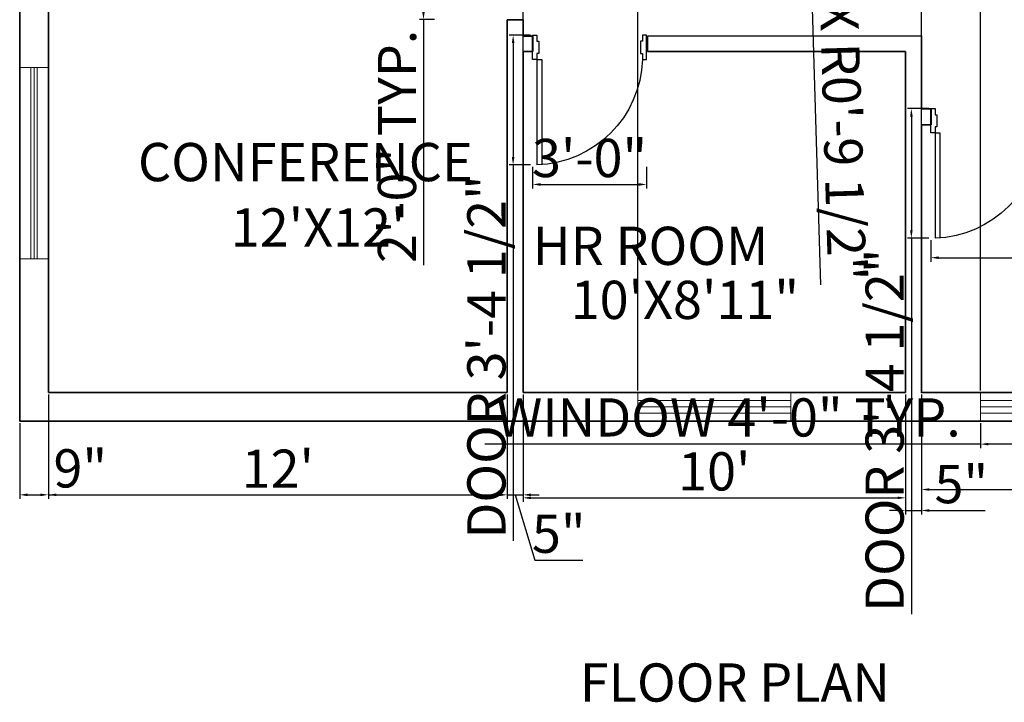
# Model space of a CAD drawing. Units: inches. Extents: x 2319 to 3765, y 2872 to 3950.
# Tile 2 of 9: x 2474 to 2783, y 2872 to 3087. Entities that reach past the tile are written whole.
import ezdxf

# ---------------------------------------------------------------- set-up
doc = ezdxf.new("R2010")
doc.units = ezdxf.units.IN
for name, color, linetype, lineweight in [('A-ANNO-DIMS', 2, 'Continuous', 18), ('A-ANNO-TEXT', 7, 'Continuous', 25), ('A-AREA-IDEN', 7, 'Continuous', 18), ('A-DOOR', 3, 'Continuous', 25), ('A-GLAZ', 4, 'Continuous', 18), ('A-WALL', 7, 'Continuous', 35)]:
    doc.layers.add(name, color=color, linetype=linetype, lineweight=lineweight)
doc.styles.get("Standard").update_dxf_attribs({"font": 'arial.ttf'})
doc.dimstyles.new('ISO-25', dxfattribs={"dimtxt": 12, "dimasz": 2.5, "dimexe": 1.25, "dimexo": 0.625, "dimtad": 1, "dimdec": 0, "dimlunit": 3, "dimtxsty": 'Standard', "dimcen": 2.5, "dimadec": 0, "dimazin": 0, "dimtfac": 1, "dimtdec": 0, "dimtmove": 0, "dimatfit": 3, "dimfxl": 1, "dimarcsym": 0})

# ---------------------------------------------------------------- blocks, each defined once
blk = doc.blocks.new('A$C769D55ED')
for p, q in [((33.6, 192), (33.6, 1024.8)), ((72, 192), (72, 1023.9)), ((0, 192), (0, 0)), ((33.6, 192), (0, 192)), ((33.6, 144), (33.6, 192)), ((48, 144), (33.6, 144)), ((48, 48), (48, 144)), ((33.6, 0), (33.6, 48)), ((33.6, 48), (48, 48)), ((0, 0), (33.6, 0))]:
    blk.add_line(p, q)
blk.add_lwpolyline([(33.6, 192), (72, 192)])
blk.add_lwpolyline([(900, 192), (900, 0), (866.4, 0), (866.4, 48), (852, 48), (852, 144), (866.4, 144), (866.4, 192)], close=True)
blk.add_arc((7.2, 165.6), 859.6, 1.76235, 88.23765)
blk = doc.blocks.new('*D20')
at = {"layer": 'A-ANNO-DIMS', "color": 0, "lineweight": -2, "transparency": 16777216}
for p, q in [((2483.13, 2968.99), (2483.13, 2936.24)), ((2627.13, 2968.99), (2627.13, 2936.24)), ((2485.63, 2937.49), (2624.63, 2937.49))]:
    blk.add_line(p, q, dxfattribs=at)
at = {"layer": 'A-ANNO-DIMS', "color": 0, "transparency": 16777216}
for points in [[(2485.63, 2937.91), (2485.63, 2937.07), (2483.13, 2937.49)], [(2624.63, 2937.91), (2624.63, 2937.07), (2627.13, 2937.49)]]:
    blk.add_solid(points, dxfattribs=at)
at = {"layer": 'Defpoints', "color": 0, "transparency": 16777216}
for p in [(2483.13, 2969.61), (2627.13, 2969.61), (2627.13, 2937.49)]:
    blk.add_point(p, dxfattribs=at)
at = {"layer": 'A-ANNO-DIMS', "color": 0, "transparency": 16777216, "insert": (2555.13, 2944.14), "char_height": 12, "attachment_point": 5}
blk.add_mtext("12'", dxfattribs=at)
blk = doc.blocks.new('*D21')
at = {"layer": 'A-ANNO-DIMS', "color": 0, "lineweight": -2, "transparency": 16777216}
for p, q in [((2632.13, 2968.99), (2632.13, 2935.3)), ((2752.13, 2968.99), (2752.13, 2935.3)), ((2634.63, 2936.55), (2749.63, 2936.55))]:
    blk.add_line(p, q, dxfattribs=at)
at = {"layer": 'A-ANNO-DIMS', "color": 0, "transparency": 16777216}
for points in [[(2634.63, 2936.96), (2634.63, 2936.13), (2632.13, 2936.55)], [(2749.63, 2936.96), (2749.63, 2936.13), (2752.13, 2936.55)]]:
    blk.add_solid(points, dxfattribs=at)
at = {"layer": 'Defpoints', "color": 0, "transparency": 16777216}
for p in [(2632.13, 2969.61), (2752.13, 2969.61), (2752.13, 2936.55)]:
    blk.add_point(p, dxfattribs=at)
at = {"layer": 'A-ANNO-DIMS', "color": 0, "transparency": 16777216, "insert": (2692.13, 2943.3), "char_height": 12, "attachment_point": 5}
blk.add_mtext("10'", dxfattribs=at)
blk = doc.blocks.new('*D22')
at = {"layer": 'A-ANNO-DIMS', "color": 0, "lineweight": -2, "transparency": 16777216}
for p, q in [((2757.13, 2968.99), (2757.13, 2937.91)), ((2946.13, 2968.99), (2946.13, 2937.91)), ((2759.63, 2939.16), (2943.63, 2939.16))]:
    blk.add_line(p, q, dxfattribs=at)
at = {"layer": 'A-ANNO-DIMS', "color": 0, "transparency": 16777216}
for points in [[(2759.63, 2939.58), (2759.63, 2938.74), (2757.13, 2939.16)], [(2943.63, 2939.58), (2943.63, 2938.74), (2946.13, 2939.16)]]:
    blk.add_solid(points, dxfattribs=at)
at = {"layer": 'Defpoints', "color": 0, "transparency": 16777216}
for p in [(2757.13, 2969.61), (2946.13, 2969.61), (2946.13, 2939.16)]:
    blk.add_point(p, dxfattribs=at)
at = {"layer": 'A-ANNO-DIMS', "color": 0, "transparency": 16777216, "insert": (2851.63, 2945.91), "char_height": 12, "attachment_point": 5}
blk.add_mtext('15\'-9"', dxfattribs=at)
blk = doc.blocks.new('*D23')
at = {"layer": 'A-ANNO-DIMS', "color": 0, "lineweight": -2, "transparency": 16777216}
for p, q in [((2474.13, 2959.99), (2474.13, 2936.24)), ((2483.13, 2951.99), (2483.13, 2936.24)), ((2476.63, 2937.49), (2480.63, 2937.49)), ((2483.13, 2937.49), (2500.67, 2937.49))]:
    blk.add_line(p, q, dxfattribs=at)
at = {"layer": 'A-ANNO-DIMS', "color": 0, "transparency": 16777216}
for points in [[(2476.63, 2937.91), (2476.63, 2937.07), (2474.13, 2937.49)], [(2480.63, 2937.91), (2480.63, 2937.07), (2483.13, 2937.49)]]:
    blk.add_solid(points, dxfattribs=at)
at = {"layer": 'Defpoints', "color": 0, "transparency": 16777216}
for p in [(2474.13, 2960.61), (2483.13, 2952.61), (2483.13, 2937.49)]:
    blk.add_point(p, dxfattribs=at)
at = {"layer": 'A-ANNO-DIMS', "color": 0, "transparency": 16777216, "insert": (2493.15, 2944.24), "char_height": 12, "attachment_point": 5}
blk.add_mtext('9"', dxfattribs=at)
blk = doc.blocks.new('*D24')
at = {"layer": 'A-ANNO-DIMS', "color": 0, "lineweight": -2, "transparency": 16777216}
for p, q in [((2627.13, 2968.99), (2627.13, 2936.24)), ((2632.13, 2968.99), (2632.13, 2936.24)), ((2624.63, 2937.49), (2622.13, 2937.49)), ((2627.13, 2937.49), (2632.13, 2937.49)), ((2627.13, 2937.49), (2632.13, 2937.49)), ((2629.63, 2937.49), (2635.78, 2916.99)), ((2634.63, 2937.49), (2637.13, 2937.49)), ((2635.78, 2916.99), (2650.82, 2916.99))]:
    blk.add_line(p, q, dxfattribs=at)
at = {"layer": 'A-ANNO-DIMS', "color": 0, "transparency": 16777216}
for points in [[(2624.63, 2937.91), (2624.63, 2937.07), (2627.13, 2937.49)], [(2634.63, 2937.91), (2634.63, 2937.07), (2632.13, 2937.49)]]:
    blk.add_solid(points, dxfattribs=at)
at = {"layer": 'Defpoints', "color": 0, "transparency": 16777216}
for p in [(2627.13, 2969.61), (2632.13, 2969.61), (2632.13, 2937.49)]:
    blk.add_point(p, dxfattribs=at)
at = {"layer": 'A-ANNO-DIMS', "color": 0, "transparency": 16777216, "insert": (2643.3, 2923.72), "char_height": 12, "attachment_point": 5}
blk.add_mtext('5"', dxfattribs=at)
blk = doc.blocks.new('*D25')
at = {"layer": 'A-ANNO-DIMS', "color": 0, "lineweight": -2, "transparency": 16777216}
for p, q in [((2752.13, 2968.99), (2752.13, 2931.32)), ((2757.13, 2968.99), (2757.13, 2931.32)), ((2749.63, 2932.57), (2747.13, 2932.57)), ((2752.13, 2932.57), (2757.13, 2932.57)), ((2759.63, 2932.57), (2777.17, 2932.57))]:
    blk.add_line(p, q, dxfattribs=at)
at = {"layer": 'A-ANNO-DIMS', "color": 0, "transparency": 16777216}
for points in [[(2749.63, 2932.99), (2749.63, 2932.15), (2752.13, 2932.57)], [(2759.63, 2932.99), (2759.63, 2932.15), (2757.13, 2932.57)]]:
    blk.add_solid(points, dxfattribs=at)
at = {"layer": 'Defpoints', "color": 0, "transparency": 16777216}
for p in [(2752.13, 2969.61), (2757.13, 2969.61), (2757.13, 2932.57)]:
    blk.add_point(p, dxfattribs=at)
at = {"layer": 'A-ANNO-DIMS', "color": 0, "transparency": 16777216, "insert": (2769.65, 2939.3), "char_height": 12, "attachment_point": 5}
blk.add_mtext('5"', dxfattribs=at)
blk = doc.blocks.new('WIN-48-PLAN-9IN-WALL')
for p, q in [((0, 9), (0, 0)), ((48, 6.5), (0, 6.5)), ((48, 9), (48, 0)), ((48, 4.5), (0, 4.5)), ((48, 2.5), (0, 2.5))]:
    blk.add_line(p, q)
blk = doc.blocks.new('*D49')
at = {"layer": 'A-ANNO-DIMS', "color": 0, "lineweight": -2, "transparency": 16777216}
for p, q in [((2634.47, 3081.78), (2627.73, 3081.78)), ((2628.98, 3079.28), (2628.98, 3043.54)), ((2634.47, 3041.04), (2627.73, 3041.04)), ((2628.98, 3041.04), (2628.98, 2923.07))]:
    blk.add_line(p, q, dxfattribs=at)
at = {"layer": 'A-ANNO-DIMS', "color": 0, "transparency": 16777216}
for points in [[(2628.57, 3079.28), (2629.4, 3079.28), (2628.98, 3081.78)], [(2628.57, 3043.54), (2629.4, 3043.54), (2628.98, 3041.04)]]:
    blk.add_solid(points, dxfattribs=at)
at = {"layer": 'Defpoints', "color": 0, "transparency": 16777216}
for p in [(2635.1, 3081.78), (2628.98, 3041.04), (2635.1, 3041.04)]:
    blk.add_point(p, dxfattribs=at)
at = {"layer": 'A-ANNO-DIMS', "color": 0, "transparency": 16777216, "insert": (2622.15, 2980.81), "char_height": 12, "attachment_point": 5, "rotation": 90}
blk.add_mtext('DOOR 3\'-4 1/2"', dxfattribs=at)
blk = doc.blocks.new('*D50')
at = {"layer": 'A-ANNO-DIMS', "color": 0, "lineweight": -2, "transparency": 16777216}
for p, q in [((2635.1, 3040.41), (2635.1, 3033.68)), ((2670.87, 3040.41), (2670.87, 3033.68)), ((2637.6, 3034.93), (2668.37, 3034.93))]:
    blk.add_line(p, q, dxfattribs=at)
at = {"layer": 'A-ANNO-DIMS', "color": 0, "transparency": 16777216}
for points in [[(2637.6, 3035.34), (2637.6, 3034.51), (2635.1, 3034.93)], [(2668.37, 3035.34), (2668.37, 3034.51), (2670.87, 3034.93)]]:
    blk.add_solid(points, dxfattribs=at)
at = {"layer": 'Defpoints', "color": 0, "transparency": 16777216}
for p in [(2635.1, 3041.04), (2670.87, 3041.04), (2670.87, 3034.93)]:
    blk.add_point(p, dxfattribs=at)
at = {"layer": 'A-ANNO-DIMS', "color": 0, "transparency": 16777216, "insert": (2652.98, 3041.68), "char_height": 12, "attachment_point": 5}
blk.add_mtext('3\'-0"', dxfattribs=at)
blk = doc.blocks.new('*D51')
at = {"layer": 'A-ANNO-DIMS', "color": 0, "lineweight": -2, "transparency": 16777216}
for p, q in [((2759.44, 3058.72), (2752.71, 3058.72)), ((2753.96, 3056.22), (2753.96, 3020.54)), ((2759.44, 3018.04), (2752.71, 3018.04)), ((2753.96, 3018.04), (2753.96, 2900.07))]:
    blk.add_line(p, q, dxfattribs=at)
at = {"layer": 'A-ANNO-DIMS', "color": 0, "transparency": 16777216}
for points in [[(2753.55, 3056.22), (2754.38, 3056.22), (2753.96, 3058.72)], [(2753.55, 3020.54), (2754.38, 3020.54), (2753.96, 3018.04)]]:
    blk.add_solid(points, dxfattribs=at)
at = {"layer": 'Defpoints', "color": 0, "transparency": 16777216}
for p in [(2760.07, 3058.72), (2753.96, 3018.04), (2760.07, 3018.04)]:
    blk.add_point(p, dxfattribs=at)
at = {"layer": 'A-ANNO-DIMS', "color": 0, "transparency": 16777216, "insert": (2747.13, 2957.8), "char_height": 12, "attachment_point": 5, "rotation": 90}
blk.add_mtext('DOOR 3\'-4 1/2"', dxfattribs=at)
blk = doc.blocks.new('*D52')
at = {"layer": 'A-ANNO-DIMS', "color": 0, "lineweight": -2, "transparency": 16777216}
for p, q in [((2760.07, 3017.41), (2760.07, 3010.68)), ((2795.8, 3017.41), (2795.8, 3010.68)), ((2762.57, 3011.93), (2793.3, 3011.93)), ((2795.8, 3011.93), (2868.94, 3011.93))]:
    blk.add_line(p, q, dxfattribs=at)
at = {"layer": 'A-ANNO-DIMS', "color": 0, "transparency": 16777216}
for points in [[(2762.57, 3012.35), (2762.57, 3011.52), (2760.07, 3011.93)], [(2793.3, 3012.35), (2793.3, 3011.52), (2795.8, 3011.93)]]:
    blk.add_solid(points, dxfattribs=at)
at = {"layer": 'Defpoints', "color": 0, "transparency": 16777216}
for p in [(2760.07, 3018.04), (2795.8, 3018.04), (2795.8, 3011.93)]:
    blk.add_point(p, dxfattribs=at)
at = {"layer": 'A-ANNO-DIMS', "color": 0, "transparency": 16777216, "insert": (2833.62, 3018.76), "char_height": 12, "attachment_point": 5}
blk.add_mtext('2\'-11 1/2"', dxfattribs=at)
blk = doc.blocks.new('*D54')
at = {"layer": 'A-ANNO-DIMS', "color": 0, "lineweight": -2, "transparency": 16777216}
for p, q in [((2604.31, 3110.61), (2599.6, 3110.61)), ((2600.85, 3108.11), (2600.85, 3089.18)), ((2604.31, 3086.68), (2599.6, 3086.68)), ((2600.85, 3086.68), (2600.85, 3009.58))]:
    blk.add_line(p, q, dxfattribs=at)
at = {"layer": 'A-ANNO-DIMS', "color": 0, "transparency": 16777216}
for points in [[(2600.43, 3108.11), (2601.26, 3108.11), (2600.85, 3110.61)], [(2600.43, 3089.18), (2601.26, 3089.18), (2600.85, 3086.68)]]:
    blk.add_solid(points, dxfattribs=at)
at = {"layer": 'Defpoints', "color": 0, "transparency": 16777216}
for p in [(2604.93, 3110.61), (2600.85, 3086.68), (2604.93, 3086.68)]:
    blk.add_point(p, dxfattribs=at)
at = {"layer": 'A-ANNO-DIMS', "color": 0, "transparency": 16777216, "insert": (2594.09, 3046.88), "char_height": 12, "attachment_point": 5, "rotation": 90}
blk.add_mtext('2\'-0" TYP.', dxfattribs=at)
blk = doc.blocks.new('*D59')
at = {"layer": 'A-ANNO-DIMS', "color": 0, "lineweight": -2, "transparency": 16777216}
for p, q in [((2775.67, 2959.99), (2775.67, 2952.16)), ((2823.67, 2959.99), (2823.67, 2952.16)), ((2775.67, 2953.41), (2620.07, 2953.41)), ((2821.17, 2953.41), (2778.17, 2953.41))]:
    blk.add_line(p, q, dxfattribs=at)
at = {"layer": 'A-ANNO-DIMS', "color": 0, "transparency": 16777216}
for points in [[(2778.17, 2953.83), (2778.17, 2952.99), (2775.67, 2953.41)], [(2821.17, 2953.83), (2821.17, 2952.99), (2823.67, 2953.41)]]:
    blk.add_solid(points, dxfattribs=at)
at = {"layer": 'Defpoints', "color": 0, "transparency": 16777216}
for p in [(2775.67, 2960.61), (2823.67, 2960.61), (2775.67, 2953.41)]:
    blk.add_point(p, dxfattribs=at)
at = {"layer": 'A-ANNO-DIMS', "color": 0, "transparency": 16777216, "insert": (2696.62, 2960.24), "char_height": 12, "attachment_point": 5}
blk.add_mtext('WINDOW 4\'-0" TYP.', dxfattribs=at)
blk = doc.blocks.new('*D75')
at = {"layer": 'A-ANNO-DIMS', "color": 0, "lineweight": -2, "transparency": 16777216}
for p, q in [((2632.13, 2970.24), (2632.13, 3605.01)), ((2634.63, 3603.76), (2665.63, 3603.76)), ((2668.13, 2970.24), (2668.13, 3605.01))]:
    blk.add_line(p, q, dxfattribs=at)
at = {"layer": 'A-ANNO-DIMS', "color": 0, "transparency": 16777216}
for points in [[(2634.63, 3604.18), (2634.63, 3603.34), (2632.13, 3603.76)], [(2665.63, 3604.18), (2665.63, 3603.34), (2668.13, 3603.76)]]:
    blk.add_solid(points, dxfattribs=at)
at = {"layer": 'Defpoints', "color": 0, "transparency": 16777216}
for p in [(2668.13, 3603.76), (2632.13, 2969.61), (2668.13, 2969.61)]:
    blk.add_point(p, dxfattribs=at)
at = {"layer": 'A-ANNO-DIMS', "color": 0, "transparency": 16777216, "insert": (2650.13, 3610.52), "char_height": 12, "attachment_point": 5}
blk.add_mtext('3\'-0"', dxfattribs=at)
blk = doc.blocks.new('*D76')
at = {"layer": 'A-ANNO-DIMS', "color": 0, "lineweight": -2, "transparency": 16777216}
for p, q in [((2757.13, 2970.24), (2757.13, 3605.01)), ((2759.63, 3603.76), (2773.17, 3603.76)), ((2775.67, 2970.24), (2775.67, 3605.01)), ((2775.67, 3603.76), (2838.15, 3603.76))]:
    blk.add_line(p, q, dxfattribs=at)
at = {"layer": 'A-ANNO-DIMS', "color": 0, "transparency": 16777216}
for points in [[(2759.63, 3604.18), (2759.63, 3603.34), (2757.13, 3603.76)], [(2773.17, 3604.18), (2773.17, 3603.34), (2775.67, 3603.76)]]:
    blk.add_solid(points, dxfattribs=at)
at = {"layer": 'Defpoints', "color": 0, "transparency": 16777216}
for p in [(2775.67, 3603.76), (2757.13, 2969.61), (2775.67, 2969.61)]:
    blk.add_point(p, dxfattribs=at)
at = {"layer": 'A-ANNO-DIMS', "color": 0, "transparency": 16777216, "insert": (2808.16, 3610.59), "char_height": 12, "attachment_point": 5}
blk.add_mtext('1\'-6 1/2"', dxfattribs=at)
blk = doc.blocks.new('*D106')
at = {"layer": 'A-ANNO-DIMS', "color": 0, "lineweight": -2, "transparency": 16777216}
for p, q in [((2721.83, 3125.82), (2722.12, 3116.28)), ((2725.52, 3003.42), (2722.2, 3113.78))]:
    blk.add_line(p, q, dxfattribs=at)
at = {"layer": 'A-ANNO-DIMS', "color": 0, "transparency": 16777216}
blk.add_solid([(2722.61, 3113.79), (2721.78, 3113.77), (2722.12, 3116.28)], dxfattribs=at)
at = {"layer": 'Defpoints', "color": 0, "transparency": 16777216}
for p in [(2721.83, 3125.82), (2722.12, 3116.28)]:
    blk.add_point(p, dxfattribs=at)
at = {"layer": 'A-ANNO-DIMS', "color": 0, "transparency": 16777216, "insert": (2730.72, 3057.56), "char_height": 12, "attachment_point": 5, "rotation": 271.7247}
blk.add_mtext('20X R0\'-9 1/2"', dxfattribs=at)

msp = doc.modelspace()

# ---------------------------------------------------------------- linework, layer by layer
at = {"layer": 'A-GLAZ'}
for p, q in [((2483.13, 3071.61), (2474.13, 3071.61)), ((2477.63, 3011.61), (2477.63, 3071.61)), ((2478.63, 3011.61), (2478.63, 3071.61)), ((2479.63, 3011.61), (2479.63, 3071.61)), ((2483.13, 3011.61), (2474.13, 3011.61)), ((2716.13, 2969.61), (2716.13, 2960.61))]:
    msp.add_line(p, q, dxfattribs=at)
at = {"layer": 'A-WALL'}
for p, q in [((2474.13, 2960.61), (2474.13, 3458.61)), ((2483.13, 2969.61), (2483.13, 3113.61)), ((2627.13, 2969.61), (2627.13, 3086.61)), ((2627.13, 3086.61), (2632.13, 3086.61)), ((2632.13, 3081.52), (2632.13, 3086.61)), ((2632.13, 3081.52), (2635.13, 3081.52)), ((2635.13, 3081.52), (2635.13, 3076.61)), ((2757.13, 3081.61), (2671.13, 3081.52)), ((2671.13, 3081.52), (2671.13, 3076.61)), ((2757.13, 3058.61), (2757.13, 3081.61)), ((2632.13, 2969.61), (2632.13, 3076.61)), ((2632.13, 3076.61), (2635.13, 3076.61)), ((2671.13, 3076.61), (2752.13, 3076.61)), ((2752.13, 2969.61), (2752.13, 3076.61)), ((2760.13, 3058.61), (2757.13, 3058.61)), ((2760.13, 3058.61), (2760.13, 3053.61)), ((2757.13, 2969.52), (2757.13, 3053.61)), ((2760.13, 3053.61), (2757.13, 3053.61)), ((2483.13, 2969.61), (2627.13, 2969.61)), ((2632.13, 2969.61), (2752.13, 2969.61)), ((2757.13, 2969.61), (2946.13, 2969.61)), ((2474.13, 2960.61), (2955.13, 2960.61))]:
    msp.add_line(p, q, dxfattribs=at)

# ---------------------------------------------------------------- block references
at = {"layer": 'A-DOOR', "rotation": 180}
for p, xscale, yscale, zscale in [((2635.1, 3081.78), -0.0397541282865356, 0.0397541282865356, 0.0397541282865356), ((2760.07, 3058.72), -0.0397016870405166, 0.0397016870405166, 0.0397016870405166)]:
    msp.add_blockref('A$C769D55ED', p, dxfattribs=dict(at, xscale=xscale, yscale=yscale, zscale=zscale))
at = {"layer": 'A-GLAZ'}
msp.add_blockref('WIN-48-PLAN-9IN-WALL', (2668.13, 2960.61), dxfattribs=at)
at = {"layer": 'A-GLAZ', "rotation": 180}
msp.add_blockref('WIN-48-PLAN-9IN-WALL', (2823.67, 2969.61), dxfattribs=at)

# ---------------------------------------------------------------- texts
at = {"layer": 'A-ANNO-TEXT'}
msp.add_text('FLOOR PLAN', height=12, dxfattribs=at).set_placement((2649.93, 2872.57))
at = {"layer": 'A-AREA-IDEN'}
for s, p in [('CONFERENCE', (2511.24, 3035.95)), ("12'X12'", (2540.38, 3015.42)), ('HR ROOM', (2635.11, 3009.66)), ('10\'X8\'11"', (2647.05, 2992.69))]:
    msp.add_text(s, height=12, dxfattribs=at).set_placement(p)

# ---------------------------------------------------------------- dimensions: what is measured, and where the dimension line sits
at = {"layer": 'A-ANNO-DIMS'}
for base, p1, p2, override, picture, middle in [((2775.67, 3603.76), (2757.13, 2969.61), (2775.67, 2969.61), {"dimdec": 1, "dimlfac": 1, "dimrnd": 0, "dimzin": 1, "dimdsep": 46, "dimlunit": 4, "dimfrac": 2}, '*D76', (2808.16, 3610.59)), ((2668.13, 3603.76), (2632.13, 2969.61), (2668.13, 2969.61), {"dimdec": 1, "dimlfac": 1, "dimrnd": 0, "dimzin": 1, "dimdsep": 46, "dimlunit": 4, "dimfrac": 2}, '*D75', (2650.13, 3610.52)), ((2670.87, 3034.93), (2635.1, 3041.04), (2670.87, 3041.04), {"dimdec": 1, "dimlfac": 1, "dimrnd": 0, "dimzin": 1, "dimdsep": 46, "dimlunit": 4, "dimfrac": 2}, '*D50', (2652.98, 3041.68)), ((2795.8, 3011.93), (2760.07, 3018.04), (2795.8, 3018.04), {"dimdec": 1, "dimlfac": 1, "dimrnd": 0, "dimzin": 1, "dimdsep": 46, "dimlunit": 4, "dimfrac": 2}, '*D52', (2833.62, 3018.76)), ((2627.13, 2937.49), (2483.13, 2969.61), (2627.13, 2969.61), {"dimclrd": 0, "dimclre": 0, "dimclrt": 0}, '*D20', (2555.13, 2944.14)), ((2632.13, 2937.49), (2627.13, 2969.61), (2632.13, 2969.61), {"dimclrd": 0, "dimclre": 0, "dimclrt": 0, "dimtmove": 1}, '*D24', (2636.4, 2923.72)), ((2752.13, 2936.55), (2632.13, 2969.61), (2752.13, 2969.61), {"dimclrd": 0, "dimclre": 0, "dimclrt": 0}, '*D21', (2692.13, 2943.3)), ((2757.13, 2932.57), (2752.13, 2969.61), (2757.13, 2969.61), {"dimclrd": 0, "dimclre": 0, "dimclrt": 0}, '*D25', (2769.65, 2939.3)), ((2946.13, 2939.16), (2757.13, 2969.61), (2946.13, 2969.61), {"dimclrd": 0, "dimclre": 0, "dimclrt": 0}, '*D22', (2851.63, 2945.91)), ((2483.13, 2937.49), (2474.13, 2960.61), (2483.13, 2952.61), {"dimclrd": 0, "dimclre": 0, "dimclrt": 0}, '*D23', (2493.15, 2944.24))]:
    dim = msp.add_linear_dim(base=base, p1=p1, p2=p2, dimstyle='ISO-25', override=override, dxfattribs=at)
    dim.commit()
    dim.dimension.update_dxf_attribs({"geometry": picture, "text_midpoint": middle})
dim = msp.add_radius_dim(center=(2721.83, 3125.82), mpoint=(2722.12, 3116.28), text='20X <>', dimstyle='ISO-25', override={"dimdec": 1, "dimlfac": 1, "dimrnd": 0, "dimzin": 1, "dimdsep": 46, "dimlunit": 4, "dimfrac": 2}, dxfattribs=at)
dim.commit()
dim.dimension.update_dxf_attribs({"geometry": '*D106', "text_midpoint": (2730.72, 3057.56)})
for base, p1, p2, angle, text, picture, middle in [((2600.85, 3086.68), (2604.93, 3110.61), (2604.93, 3086.68), 270, '<> TYP.', '*D54', (2594.09, 3046.88)), ((2628.98, 3041.04), (2635.1, 3081.78), (2635.1, 3041.04), 270, 'DOOR <>', '*D49', (2622.15, 2980.81)), ((2753.96, 3018.04), (2760.07, 3058.72), (2760.07, 3018.04), 270, 'DOOR <>', '*D51', (2747.13, 2957.8)), ((2775.67, 2953.41), (2823.67, 2960.61), (2775.67, 2960.61), 180, 'WINDOW <> TYP.', '*D59', (2696.62, 2960.24))]:
    dim = msp.add_linear_dim(base=base, p1=p1, p2=p2, angle=angle, text=text, dimstyle='ISO-25', override={"dimdec": 1, "dimlfac": 1, "dimrnd": 0, "dimzin": 1, "dimdsep": 46, "dimlunit": 4, "dimfrac": 2}, dxfattribs=at)
    dim.commit()
    dim.dimension.update_dxf_attribs({"geometry": picture, "text_midpoint": middle})

doc.saveas('drawing.dxf')
